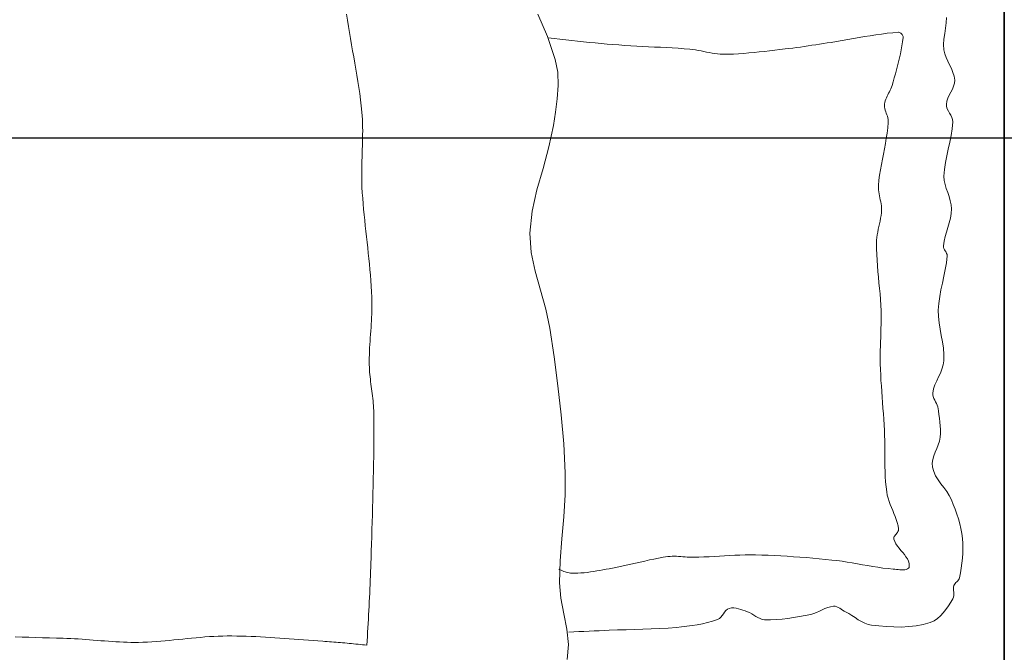
# Model space of a CAD drawing. Units: inches. Extents: x 1484 to 2008, y 1843 to 2590.
# Tile 6 of 21: x 1853 to 1891, y 1981 to 2005. Entities that reach past the tile are written whole.
import ezdxf

# ---------------------------------------------------------------- set-up
doc = ezdxf.new("R2010")
doc.units = ezdxf.units.IN
for name, color, linetype, lineweight in [('A-ANNO-DIMS', 2, 'Continuous', 18), ('A-FURN', 8, 'Continuous', 18), ('A-WALL', 7, 'Continuous', 35)]:
    doc.layers.add(name, color=color, linetype=linetype, lineweight=lineweight)
doc.styles.get("Standard").update_dxf_attribs({"font": 'arial.ttf'})
doc.dimstyles.new('ISO-25', dxfattribs={"dimtxt": 7, "dimasz": 2.5, "dimexe": 1.25, "dimexo": 0.625, "dimtad": 1, "dimdec": 0, "dimlunit": 3, "dimtxsty": 'Standard', "dimcen": 2.5, "dimadec": 0, "dimazin": 0, "dimtfac": 1, "dimtdec": 0, "dimtmove": 0, "dimatfit": 3, "dimfxl": 1, "dimarcsym": 0})

# ---------------------------------------------------------------- blocks, each defined once
blk = doc.blocks.new('BED-DOUBLE')
for p, q in [((48.589, 84.891), (48.4, 84.837)), ((48.78, 84.936), (48.589, 84.891)), ((48.973, 84.972), (48.78, 84.936)), ((49.167, 84.998), (48.973, 84.972)), ((49.359, 85.013), (49.167, 84.998)), ((49.551, 85.017), (49.359, 85.013)), ((49.744, 85.011), (49.551, 85.017)), ((49.937, 84.997), (49.744, 85.011)), ((50.129, 84.977), (49.937, 84.997)), ((50.321, 84.951), (50.129, 84.977)), ((50.512, 84.921), (50.321, 84.951)), ((50.702, 84.887), (50.512, 84.921)), ((50.746, 84.873), (50.702, 84.887)), ((50.784, 84.848), (50.746, 84.873)), ((50.82, 84.817), (50.784, 84.848)), ((30.689, 84.496), (30.546, 84.424)), ((30.832, 84.567), (30.689, 84.496)), ((30.977, 84.628), (30.832, 84.567)), ((31.125, 84.673), (30.977, 84.628)), ((31.278, 84.695), (31.125, 84.673)), ((31.401, 84.686), (31.278, 84.695)), ((31.52, 84.653), (31.401, 84.686)), ((31.637, 84.603), (31.52, 84.653)), ((31.752, 84.545), (31.637, 84.603)), ((31.867, 84.485), (31.752, 84.545)), ((31.984, 84.431), (31.867, 84.485)), ((32.569, 84.494), (32.485, 84.447)), ((32.652, 84.541), (32.569, 84.494)), ((32.736, 84.582), (32.652, 84.541)), ((32.822, 84.61), (32.736, 84.582)), ((32.912, 84.619), (32.822, 84.61)), ((33.179, 84.598), (32.912, 84.619)), ((33.443, 84.556), (33.179, 84.598)), ((33.707, 84.502), (33.443, 84.556)), ((33.97, 84.442), (33.707, 84.502)), ((35.826, 84.476), (35.668, 84.421)), ((35.985, 84.524), (35.826, 84.476)), ((36.145, 84.558), (35.985, 84.524)), ((36.307, 84.57), (36.145, 84.558)), ((36.49, 84.557), (36.307, 84.57)), ((36.671, 84.526), (36.49, 84.557)), ((36.85, 84.482), (36.671, 84.526)), ((37.029, 84.43), (36.85, 84.482)), ((47.495, 84.483), (47.337, 84.382)), ((47.661, 84.566), (47.495, 84.483)), ((47.843, 84.64), (47.661, 84.566)), ((48.027, 84.711), (47.843, 84.64)), ((48.212, 84.777), (48.027, 84.711)), ((48.4, 84.837), (48.212, 84.777)), ((50.855, 84.782), (50.82, 84.817)), ((50.889, 84.745), (50.855, 84.782)), ((50.924, 84.712), (50.889, 84.745)), ((50.962, 84.684), (50.924, 84.712)), ((51.004, 84.664), (50.962, 84.684)), ((51.067, 84.651), (51.004, 84.664)), ((51.133, 84.649), (51.067, 84.651)), ((51.2, 84.654), (51.133, 84.649)), ((51.267, 84.661), (51.2, 84.654)), ((51.334, 84.665), (51.267, 84.661)), ((51.398, 84.664), (51.334, 84.665)), ((51.459, 84.653), (51.398, 84.664)), ((51.516, 84.627), (51.459, 84.653)), ((51.654, 84.54), (51.516, 84.627)), ((51.794, 84.449), (51.654, 84.54)), ((29.039, 84.367), (28.83, 84.378)), ((29.252, 84.339), (29.039, 84.367)), ((29.466, 84.304), (29.252, 84.339)), ((29.68, 84.274), (29.466, 84.304)), ((29.893, 84.259), (29.68, 84.274)), ((30.102, 84.27), (29.893, 84.259)), ((30.254, 84.304), (30.102, 84.27)), ((30.402, 84.358), (30.254, 84.304)), ((30.546, 84.424), (30.402, 84.358)), ((32.103, 84.39), (31.984, 84.431)), ((32.226, 84.372), (32.103, 84.39)), ((32.315, 84.379), (32.226, 84.372)), ((32.401, 84.407), (32.315, 84.379)), ((32.485, 84.447), (32.401, 84.407)), ((34.233, 84.382), (33.97, 84.442)), ((34.497, 84.33), (34.233, 84.382)), ((34.762, 84.292), (34.497, 84.33)), ((35.029, 84.275), (34.762, 84.292)), ((35.192, 84.286), (35.029, 84.275)), ((35.352, 84.319), (35.192, 84.286)), ((35.511, 84.366), (35.352, 84.319)), ((35.668, 84.421), (35.511, 84.366)), ((37.207, 84.376), (37.029, 84.43)), ((37.386, 84.326), (37.207, 84.376)), ((37.566, 84.285), (37.386, 84.326)), ((37.749, 84.259), (37.566, 84.285)), ((37.8, 84.262), (37.749, 84.259)), ((37.849, 84.277), (37.8, 84.262)), ((37.897, 84.301), (37.849, 84.277)), ((37.945, 84.329), (37.897, 84.301)), ((37.992, 84.357), (37.945, 84.329)), ((38.04, 84.381), (37.992, 84.357)), ((38.09, 84.397), (38.04, 84.381)), ((38.141, 84.4), (38.09, 84.397)), ((38.407, 84.37), (38.141, 84.4)), ((38.672, 84.325), (38.407, 84.37)), ((38.936, 84.272), (38.672, 84.325)), ((39.199, 84.215), (38.936, 84.272)), ((39.462, 84.16), (39.199, 84.215)), ((39.726, 84.112), (39.462, 84.16)), ((39.991, 84.075), (39.726, 84.112)), ((40.258, 84.056), (39.991, 84.075)), ((40.753, 84.087), (40.506, 84.061)), ((40.999, 84.126), (40.753, 84.087)), ((41.245, 84.171), (40.999, 84.126)), ((41.491, 84.216), (41.245, 84.171)), ((41.737, 84.252), (41.491, 84.216)), ((41.984, 84.272), (41.737, 84.252)), ((42.231, 84.269), (41.984, 84.272)), ((42.394, 84.244), (42.231, 84.269)), ((42.553, 84.197), (42.394, 84.244)), ((42.709, 84.135), (42.553, 84.197)), ((42.863, 84.064), (42.709, 84.135)), ((44.327, 84.08), (44.179, 84.057)), ((44.475, 84.101), (44.327, 84.08)), ((44.623, 84.118), (44.475, 84.101)), ((44.772, 84.13), (44.623, 84.118)), ((44.92, 84.137), (44.772, 84.13)), ((45.069, 84.136), (44.92, 84.137)), ((45.217, 84.128), (45.069, 84.136)), ((45.365, 84.102), (45.217, 84.128)), ((45.511, 84.056), (45.365, 84.102)), ((47.031, 84.157), (46.877, 84.048)), ((47.183, 84.271), (47.031, 84.157)), ((47.337, 84.382), (47.183, 84.271)), ((51.933, 84.353), (51.794, 84.449)), ((52.065, 84.251), (51.933, 84.353)), ((52.187, 84.141), (52.065, 84.251)), ((52.294, 84.02), (52.187, 84.141)), ((40.506, 84.061), (40.258, 84.056)), ((43.017, 83.992), (42.863, 84.064)), ((43.173, 83.926), (43.017, 83.992)), ((43.331, 83.872), (43.173, 83.926)), ((43.493, 83.838), (43.331, 83.872)), ((43.563, 83.838), (43.493, 83.838)), ((43.631, 83.854), (43.563, 83.838)), ((43.698, 83.881), (43.631, 83.854)), ((43.763, 83.914), (43.698, 83.881)), ((43.829, 83.951), (43.763, 83.914)), ((43.896, 83.986), (43.829, 83.951)), ((43.963, 84.014), (43.896, 83.986)), ((44.033, 84.033), (43.963, 84.014)), ((44.179, 84.057), (44.033, 84.033)), ((45.655, 83.998), (45.511, 84.056)), ((45.799, 83.937), (45.655, 83.998)), ((45.942, 83.881), (45.799, 83.937)), ((46.086, 83.839), (45.942, 83.881)), ((46.231, 83.818), (46.086, 83.839)), ((46.378, 83.826), (46.231, 83.818)), ((46.554, 83.875), (46.378, 83.826)), ((46.719, 83.952), (46.554, 83.875)), ((46.877, 84.048), (46.719, 83.952)), ((52.381, 83.888), (52.294, 84.02)), ((52.444, 83.743), (52.381, 83.888)), ((52.52, 83.468), (52.444, 83.743)), ((52.573, 83.186), (52.52, 83.468)), ((50.149, 82.915), (50.247, 82.924)), ((50.247, 82.924), (50.294, 82.915)), ((52.606, 82.9), (52.573, 83.186)), ((29.413, 82.522), (29.419, 82.546)), ((29.419, 82.546), (29.429, 82.569)), ((29.429, 82.569), (29.443, 82.591)), ((29.443, 82.591), (29.46, 82.612)), ((29.46, 82.612), (29.48, 82.631)), ((29.48, 82.631), (29.502, 82.648)), ((29.502, 82.648), (29.525, 82.662)), ((29.525, 82.662), (29.549, 82.674)), ((29.549, 82.674), (29.574, 82.681)), ((29.574, 82.681), (29.598, 82.685)), ((29.598, 82.685), (29.622, 82.685)), ((29.622, 82.685), (29.781, 82.664)), ((29.781, 82.664), (29.939, 82.639)), ((29.939, 82.639), (30.096, 82.61)), ((30.096, 82.61), (30.253, 82.578)), ((30.253, 82.578), (30.409, 82.543)), ((30.409, 82.543), (30.565, 82.506)), ((49.548, 82.528), (49.631, 82.597)), ((49.631, 82.597), (49.713, 82.667)), ((49.713, 82.667), (49.796, 82.734)), ((49.796, 82.734), (49.88, 82.795)), ((49.88, 82.795), (49.966, 82.848)), ((49.966, 82.848), (50.055, 82.889)), ((50.055, 82.889), (50.149, 82.915)), ((50.294, 82.915), (50.33, 82.891)), ((50.33, 82.891), (50.357, 82.854)), ((50.357, 82.854), (50.374, 82.807)), ((50.374, 82.807), (50.385, 82.751)), ((50.386, 82.555), (50.38, 82.486)), ((50.385, 82.751), (50.39, 82.689)), ((50.39, 82.623), (50.386, 82.555)), ((50.39, 82.689), (50.39, 82.623)), ((52.621, 82.611), (52.606, 82.9)), ((52.62, 82.321), (52.621, 82.611)), ((29.412, 82.499), (29.413, 82.522)), ((29.429, 82.278), (29.412, 82.499)), ((29.452, 82.058), (29.429, 82.278)), ((30.565, 82.506), (30.721, 82.466)), ((30.721, 82.466), (30.876, 82.425)), ((30.876, 82.425), (31.031, 82.383)), ((31.031, 82.383), (31.186, 82.34)), ((31.186, 82.34), (31.34, 82.296)), ((31.34, 82.296), (31.494, 82.253)), ((31.494, 82.253), (31.556, 82.233)), ((31.556, 82.233), (31.616, 82.208)), ((31.616, 82.208), (31.675, 82.181)), ((31.675, 82.181), (31.733, 82.151)), ((47.717, 82.138), (47.836, 82.181)), ((47.836, 82.181), (47.954, 82.228)), ((47.954, 82.228), (48.072, 82.276)), ((48.072, 82.276), (48.189, 82.325)), ((48.189, 82.325), (48.307, 82.372)), ((48.307, 82.372), (48.426, 82.415)), ((48.426, 82.415), (48.546, 82.454)), ((48.546, 82.454), (48.667, 82.486)), ((48.667, 82.486), (48.791, 82.509)), ((48.791, 82.509), (48.827, 82.509)), ((48.827, 82.509), (48.861, 82.5)), ((48.861, 82.5), (48.895, 82.483)), ((48.895, 82.483), (48.928, 82.461)), ((48.928, 82.461), (48.96, 82.435)), ((48.96, 82.435), (48.992, 82.408)), ((48.992, 82.408), (49.024, 82.381)), ((49.024, 82.381), (49.057, 82.357)), ((49.057, 82.357), (49.089, 82.336)), ((49.089, 82.336), (49.122, 82.323)), ((49.122, 82.323), (49.156, 82.317)), ((49.156, 82.317), (49.191, 82.321)), ((49.191, 82.321), (49.286, 82.356)), ((49.286, 82.356), (49.376, 82.405)), ((49.376, 82.405), (49.463, 82.463)), ((49.463, 82.463), (49.548, 82.528)), ((50.361, 82.3), (50.343, 82.099)), ((50.367, 82.357), (50.361, 82.3)), ((50.373, 82.419), (50.367, 82.357)), ((50.38, 82.486), (50.373, 82.419)), ((52.606, 82.03), (52.62, 82.321)), ((29.48, 81.839), (29.452, 82.058)), ((29.511, 81.62), (29.48, 81.839)), ((31.733, 82.151), (31.791, 82.12)), ((31.791, 82.12), (31.849, 82.088)), ((31.849, 82.088), (31.907, 82.058)), ((31.907, 82.058), (31.966, 82.03)), ((31.966, 82.03), (32.025, 82.004)), ((32.025, 82.004), (32.085, 81.983)), ((32.085, 81.983), (32.147, 81.967)), ((32.147, 81.967), (32.21, 81.957)), ((32.21, 81.957), (32.271, 81.955)), ((32.271, 81.955), (32.331, 81.961)), ((32.331, 81.961), (32.392, 81.972)), ((32.392, 81.972), (32.451, 81.989)), ((32.451, 81.989), (32.511, 82.008)), ((32.511, 82.008), (32.571, 82.029)), ((32.571, 82.029), (32.63, 82.05)), ((32.63, 82.05), (32.69, 82.07)), ((32.69, 82.07), (32.75, 82.087)), ((32.75, 82.087), (32.81, 82.1)), ((32.81, 82.1), (32.871, 82.107)), ((32.871, 82.107), (32.932, 82.106)), ((32.932, 82.106), (33.138, 82.087)), ((33.138, 82.087), (33.345, 82.061)), ((33.345, 82.061), (33.55, 82.029)), ((33.55, 82.029), (33.755, 81.994)), ((33.755, 81.994), (33.96, 81.955)), ((33.96, 81.955), (34.164, 81.915)), ((34.164, 81.915), (34.369, 81.875)), ((34.369, 81.875), (34.573, 81.836)), ((34.573, 81.836), (34.778, 81.8)), ((34.778, 81.8), (34.983, 81.768)), ((34.983, 81.768), (35.189, 81.741)), ((35.793, 81.76), (35.872, 81.777)), ((35.872, 81.777), (35.952, 81.795)), ((35.952, 81.795), (36.031, 81.811)), ((36.031, 81.811), (36.11, 81.826)), ((36.11, 81.826), (36.19, 81.837)), ((36.19, 81.837), (36.269, 81.843)), ((36.269, 81.843), (36.349, 81.844)), ((36.349, 81.844), (36.458, 81.837)), ((36.458, 81.837), (36.565, 81.824)), ((36.565, 81.824), (36.673, 81.806)), ((36.673, 81.806), (36.78, 81.786)), ((36.78, 81.786), (36.887, 81.763)), ((39.405, 81.764), (39.625, 81.784)), ((39.625, 81.784), (39.846, 81.801)), ((39.846, 81.801), (40.067, 81.815)), ((40.067, 81.815), (40.288, 81.824)), ((40.288, 81.824), (40.46, 81.828)), ((40.46, 81.828), (40.631, 81.828)), ((40.631, 81.828), (40.803, 81.825)), ((40.803, 81.825), (40.975, 81.821)), ((40.975, 81.821), (41.147, 81.815)), ((41.147, 81.815), (41.318, 81.809)), ((41.318, 81.809), (41.49, 81.802)), ((41.49, 81.802), (41.662, 81.797)), ((41.662, 81.797), (41.834, 81.792)), ((41.834, 81.792), (42.005, 81.789)), ((42.005, 81.789), (42.177, 81.789)), ((42.177, 81.789), (42.349, 81.792)), ((42.349, 81.792), (42.566, 81.799)), ((42.566, 81.799), (42.782, 81.809)), ((42.782, 81.809), (42.999, 81.821)), ((42.999, 81.821), (43.216, 81.835)), ((43.216, 81.835), (43.432, 81.85)), ((43.432, 81.85), (43.649, 81.866)), ((43.649, 81.866), (43.865, 81.882)), ((43.865, 81.882), (44.082, 81.898)), ((44.082, 81.898), (44.298, 81.914)), ((44.298, 81.914), (44.515, 81.928)), ((44.515, 81.928), (44.732, 81.942)), ((44.732, 81.942), (44.948, 81.954)), ((44.948, 81.954), (45.149, 81.962)), ((45.149, 81.962), (45.349, 81.967)), ((45.349, 81.967), (45.55, 81.969)), ((45.55, 81.969), (45.751, 81.97)), ((45.751, 81.97), (45.952, 81.971)), ((45.952, 81.971), (46.153, 81.972)), ((46.153, 81.972), (46.354, 81.975)), ((46.354, 81.975), (46.554, 81.98)), ((46.554, 81.98), (46.754, 81.989)), ((46.754, 81.989), (46.954, 82.002)), ((46.954, 82.002), (47.153, 82.02)), ((47.153, 82.02), (47.352, 82.046)), ((47.352, 82.046), (47.476, 82.068)), ((47.476, 82.068), (47.597, 82.1)), ((47.597, 82.1), (47.717, 82.138)), ((50.319, 81.899), (50.291, 81.699)), ((50.343, 82.099), (50.319, 81.899)), ((52.581, 81.741), (52.606, 82.03)), ((29.545, 81.401), (29.511, 81.62)), ((29.582, 81.182), (29.545, 81.401)), ((35.189, 81.741), (35.396, 81.722)), ((35.396, 81.722), (35.476, 81.719)), ((35.476, 81.719), (35.555, 81.723)), ((35.555, 81.723), (35.635, 81.732)), ((35.635, 81.732), (35.714, 81.745)), ((35.714, 81.745), (35.793, 81.76)), ((36.887, 81.763), (36.994, 81.739)), ((36.994, 81.739), (37.101, 81.716)), ((37.101, 81.716), (37.208, 81.694)), ((37.208, 81.694), (37.315, 81.674)), ((37.315, 81.674), (37.423, 81.659)), ((37.423, 81.659), (37.531, 81.648)), ((37.531, 81.648), (37.639, 81.644)), ((37.639, 81.644), (37.86, 81.646)), ((37.86, 81.646), (38.081, 81.654)), ((38.081, 81.654), (38.302, 81.667)), ((38.302, 81.667), (38.523, 81.683)), ((38.523, 81.683), (38.743, 81.702)), ((38.743, 81.702), (38.964, 81.722)), ((38.964, 81.722), (39.184, 81.743)), ((39.184, 81.743), (39.405, 81.764)), ((50.26, 81.499), (50.226, 81.3)), ((50.291, 81.699), (50.26, 81.499)), ((52.52, 81.317), (52.549, 81.455)), ((52.549, 81.455), (52.581, 81.741)), ((29.62, 80.964), (29.582, 81.182)), ((50.192, 81.1), (50.157, 80.901)), ((50.226, 81.3), (50.192, 81.1)), ((52.335, 80.933), (52.409, 81.057)), ((52.409, 81.057), (52.472, 81.185)), ((52.472, 81.185), (52.52, 81.317)), ((29.659, 80.746), (29.62, 80.964)), ((29.698, 80.527), (29.659, 80.746)), ((50.122, 80.702), (50.089, 80.503)), ((50.157, 80.901), (50.122, 80.702)), ((52.099, 80.564), (52.176, 80.687)), ((52.176, 80.687), (52.256, 80.81)), ((52.256, 80.81), (52.335, 80.933)), ((29.736, 80.309), (29.698, 80.527)), ((29.772, 80.09), (29.736, 80.309)), ((50.058, 80.303), (50.031, 80.103)), ((50.089, 80.503), (50.058, 80.303)), ((51.887, 80.211), (51.924, 80.267)), ((51.924, 80.267), (51.962, 80.324)), ((51.962, 80.324), (51.998, 80.38)), ((51.998, 80.38), (52.03, 80.437)), ((52.03, 80.437), (52.099, 80.564)), ((29.806, 79.872), (29.772, 80.09)), ((29.828, 79.723), (29.806, 79.872)), ((50.008, 79.902), (49.983, 79.654)), ((50.031, 80.103), (50.008, 79.902)), ((51.811, 79.971), (51.813, 80.034)), ((51.828, 79.856), (51.811, 79.971)), ((51.813, 80.034), (51.829, 80.094)), ((51.861, 79.744), (51.828, 79.856)), ((51.829, 80.094), (51.854, 80.153)), ((51.854, 80.153), (51.887, 80.211)), ((29.851, 79.574), (29.828, 79.723)), ((29.874, 79.425), (29.851, 79.574)), ((49.983, 79.654), (49.959, 79.407)), ((51.905, 79.636), (51.861, 79.744)), ((51.956, 79.528), (51.905, 79.636)), ((52.008, 79.42), (51.956, 79.528)), ((29.897, 79.276), (29.874, 79.425)), ((29.92, 79.127), (29.897, 79.276)), ((29.943, 78.978), (29.92, 79.127)), ((49.937, 79.159), (49.915, 78.911)), ((49.959, 79.407), (49.937, 79.159)), ((52.057, 79.312), (52.008, 79.42)), ((52.099, 79.202), (52.057, 79.312)), ((52.129, 79.089), (52.099, 79.202)), ((52.172, 78.865), (52.129, 79.089)), ((29.965, 78.829), (29.943, 78.978)), ((29.987, 78.679), (29.965, 78.829)), ((49.915, 78.911), (49.896, 78.663)), ((52.214, 78.64), (52.172, 78.865)), ((30.008, 78.53), (29.987, 78.679)), ((30.027, 78.381), (30.008, 78.53)), ((30.046, 78.231), (30.027, 78.381)), ((49.877, 78.414), (49.861, 78.166)), ((49.896, 78.663), (49.877, 78.414)), ((52.253, 78.415), (52.214, 78.64)), ((52.286, 78.189), (52.253, 78.415)), ((30.063, 78.082), (30.046, 78.231)), ((30.086, 77.881), (30.063, 78.082)), ((49.861, 78.166), (49.846, 77.917)), ((52.313, 77.962), (52.286, 78.189)), ((52.332, 77.735), (52.313, 77.962)), ((30.11, 77.68), (30.086, 77.881)), ((30.133, 77.479), (30.11, 77.68)), ((49.834, 77.669), (49.823, 77.42)), ((49.846, 77.917), (49.834, 77.669)), ((52.341, 77.508), (52.332, 77.735)), ((30.156, 77.277), (30.133, 77.479)), ((30.179, 77.076), (30.156, 77.277)), ((49.815, 77.172), (49.808, 76.923)), ((49.823, 77.42), (49.815, 77.172)), ((52.295, 77.106), (52.324, 77.192)), ((52.324, 77.192), (52.337, 77.281)), ((52.337, 77.281), (52.341, 77.508)), ((30.2, 76.875), (30.179, 77.076)), ((30.219, 76.673), (30.2, 76.875)), ((49.808, 76.923), (49.807, 76.722)), ((52.059, 76.7), (52.103, 76.783)), ((52.103, 76.783), (52.154, 76.863)), ((52.154, 76.863), (52.205, 76.943)), ((52.205, 76.943), (52.254, 77.024)), ((52.254, 77.024), (52.295, 77.106)), ((30.236, 76.472), (30.219, 76.673)), ((30.25, 76.27), (30.236, 76.472)), ((49.807, 76.722), (49.809, 76.522)), ((49.809, 76.522), (49.814, 76.322)), ((51.934, 76.35), (51.964, 76.439)), ((51.964, 76.439), (51.995, 76.527)), ((51.995, 76.527), (52.024, 76.614)), ((52.024, 76.614), (52.059, 76.7)), ((30.261, 76.068), (30.25, 76.27)), ((30.268, 75.866), (30.261, 76.068)), ((49.814, 76.322), (49.822, 76.122)), ((49.822, 76.122), (49.831, 75.921)), ((51.877, 76.08), (51.888, 76.17)), ((51.878, 75.991), (51.877, 76.08)), ((51.888, 76.17), (51.908, 76.26)), ((51.908, 76.26), (51.934, 76.35)), ((30.271, 75.664), (30.268, 75.866)), ((30.268, 75.556), (30.271, 75.664)), ((49.831, 75.921), (49.842, 75.721)), ((49.842, 75.721), (49.854, 75.521)), ((51.893, 75.902), (51.878, 75.991)), ((51.925, 75.833), (51.893, 75.902)), ((51.974, 75.774), (51.925, 75.833)), ((52.037, 75.723), (51.974, 75.774)), ((52.106, 75.675), (52.037, 75.723)), ((52.176, 75.628), (52.106, 75.675)), ((52.241, 75.577), (52.176, 75.628)), ((30.228, 75.233), (30.245, 75.34)), ((30.245, 75.34), (30.259, 75.448)), ((30.259, 75.448), (30.268, 75.556)), ((49.854, 75.521), (49.866, 75.32)), ((49.866, 75.32), (49.877, 75.12)), ((52.295, 75.519), (52.241, 75.577)), ((52.333, 75.452), (52.295, 75.519)), ((52.397, 75.258), (52.333, 75.452)), ((52.45, 75.06), (52.397, 75.258)), ((30.14, 74.805), (30.163, 74.912)), ((30.163, 74.912), (30.186, 75.019)), ((30.186, 75.019), (30.208, 75.126)), ((30.208, 75.126), (30.228, 75.233)), ((49.877, 75.12), (49.887, 74.92)), ((49.887, 74.92), (49.895, 74.72)), ((52.496, 74.861), (52.45, 75.06)), ((52.533, 74.659), (52.496, 74.861)), ((30.071, 74.374), (30.083, 74.482)), ((30.083, 74.482), (30.1, 74.59)), ((30.1, 74.59), (30.119, 74.697)), ((30.119, 74.697), (30.14, 74.805)), ((49.895, 74.72), (49.9, 74.519)), ((49.9, 74.519), (49.9, 74.435)), ((52.565, 74.456), (52.533, 74.659)), ((30.036, 73.913), (30.052, 74.144)), ((30.052, 74.144), (30.071, 74.374)), ((49.88, 74.099), (49.873, 74.015)), ((49.887, 74.183), (49.88, 74.099)), ((49.893, 74.267), (49.887, 74.183)), ((49.897, 74.351), (49.893, 74.267)), ((49.9, 74.435), (49.897, 74.351)), ((52.592, 74.252), (52.565, 74.456)), ((52.615, 74.048), (52.592, 74.252)), ((30.021, 73.682), (30.036, 73.913)), ((49.863, 73.847), (49.861, 73.764)), ((49.861, 73.764), (49.862, 73.68)), ((49.868, 73.931), (49.863, 73.847)), ((49.873, 74.015), (49.868, 73.931)), ((52.635, 73.844), (52.615, 74.048)), ((52.663, 73.518), (52.635, 73.844)), ((29.997, 73.219), (30.009, 73.451)), ((30.009, 73.451), (30.021, 73.682)), ((49.862, 73.68), (49.866, 73.597)), ((49.866, 73.597), (49.875, 73.513)), ((49.875, 73.513), (49.902, 73.331)), ((49.902, 73.331), (49.933, 73.15)), ((52.684, 73.191), (52.663, 73.518)), ((29.976, 72.757), (29.987, 72.988)), ((29.987, 72.988), (29.997, 73.219)), ((49.933, 73.15), (49.968, 72.969)), ((49.968, 72.969), (50.006, 72.789)), ((52.699, 72.864), (52.684, 73.191)), ((29.965, 72.526), (29.976, 72.757)), ((50.006, 72.789), (50.046, 72.609)), ((50.046, 72.609), (50.087, 72.429)), ((52.71, 72.537), (52.699, 72.864)), ((29.94, 72.063), (29.953, 72.295)), ((29.953, 72.295), (29.965, 72.526)), ((50.087, 72.429), (50.129, 72.25)), ((50.129, 72.25), (50.171, 72.07)), ((52.718, 72.209), (52.71, 72.537)), ((52.727, 71.882), (52.718, 72.209)), ((29.908, 71.602), (29.925, 71.833)), ((29.925, 71.833), (29.94, 72.063)), ((50.171, 72.07), (50.212, 71.891)), ((50.212, 71.891), (50.252, 71.711)), ((52.736, 71.554), (52.727, 71.882)), ((29.889, 71.371), (29.908, 71.602)), ((50.252, 71.711), (50.289, 71.53)), ((50.289, 71.53), (50.323, 71.349)), ((52.749, 71.227), (52.736, 71.554)), ((29.849, 70.911), (29.87, 71.141)), ((29.87, 71.141), (29.889, 71.371)), ((50.323, 71.349), (50.345, 71.227)), ((50.345, 71.227), (50.368, 71.104)), ((50.368, 71.104), (50.39, 70.982)), ((52.757, 71.029), (52.749, 71.227)), ((52.766, 70.832), (52.757, 71.029)), ((29.806, 70.451), (29.828, 70.681)), ((29.828, 70.681), (29.849, 70.911)), ((50.39, 70.982), (50.412, 70.859)), ((50.412, 70.859), (50.433, 70.736)), ((50.433, 70.736), (50.453, 70.613)), ((52.775, 70.634), (52.766, 70.832)), ((29.783, 70.221), (29.806, 70.451)), ((50.453, 70.613), (50.471, 70.49)), ((50.471, 70.49), (50.488, 70.366)), ((50.488, 70.366), (50.501, 70.243)), ((52.784, 70.437), (52.775, 70.634)), ((52.793, 70.239), (52.784, 70.437)), ((29.735, 69.761), (29.76, 69.991)), ((29.76, 69.991), (29.783, 70.221)), ((50.501, 70.243), (50.512, 70.119)), ((50.512, 70.119), (50.52, 69.995)), ((50.52, 69.995), (50.524, 69.871)), ((50.524, 69.871), (50.524, 69.818)), ((52.802, 70.042), (52.793, 70.239)), ((52.811, 69.844), (52.802, 70.042)), ((29.684, 69.302), (29.71, 69.532)), ((29.71, 69.532), (29.735, 69.761)), ((46.611, 69.512), (45.475, 69.449)), ((47.469, 69.508), (46.611, 69.512)), ((48.327, 69.451), (47.469, 69.508)), ((50.468, 69.501), (50.45, 69.45)), ((50.483, 69.552), (50.468, 69.501)), ((50.496, 69.605), (50.483, 69.552)), ((50.507, 69.658), (50.496, 69.605)), ((50.515, 69.711), (50.507, 69.658)), ((50.521, 69.764), (50.515, 69.711)), ((50.524, 69.818), (50.521, 69.764)), ((52.703, 69.567), (52.103, 69.452)), ((53.299, 69.631), (52.703, 69.567)), ((52.82, 69.647), (52.811, 69.844)), ((53.892, 69.59), (53.299, 69.631)), ((30.471, 69.119), (29.579, 68.813)), ((29.657, 69.072), (29.684, 69.302)), ((30.973, 69.217), (30.471, 69.119)), ((31.488, 69.235), (30.973, 69.217)), ((32.008, 69.198), (31.488, 69.235)), ((32.529, 69.128), (32.008, 69.198)), ((33.044, 69.05), (32.529, 69.128)), ((43.211, 69.223), (42.083, 69.075)), ((44.342, 69.35), (43.211, 69.223)), ((45.475, 69.449), (44.342, 69.35)), ((49.184, 69.375), (48.327, 69.451)), ((50.042, 69.309), (49.184, 69.375)), ((50.901, 69.287), (50.042, 69.309)), ((50.384, 69.303), (50.358, 69.257)), ((50.408, 69.351), (50.384, 69.303)), ((50.431, 69.4), (50.408, 69.351)), ((50.45, 69.45), (50.431, 69.4)), ((51.502, 69.34), (50.901, 69.287)), ((52.103, 69.452), (51.502, 69.34)), ((29.579, 68.813), (28.71, 68.44)), ((29.629, 68.843), (29.657, 69.072)), ((33.889, 68.877), (33.044, 69.05)), ((34.725, 68.644), (33.889, 68.877)), ((40.213, 68.759), (39.476, 68.552)), ((40.957, 68.913), (40.213, 68.759)), ((42.083, 69.075), (40.957, 68.913)), ((35.559, 68.405), (34.725, 68.644)), ((36.399, 68.216), (35.559, 68.405)), ((38.741, 68.343), (38.002, 68.186)), ((39.476, 68.552), (38.741, 68.343)), ((37.252, 68.131), (36.399, 68.216)), ((38.002, 68.186), (37.252, 68.131)), ((37.818, 61.809), (37.604, 61.785)), ((38.032, 61.832), (37.818, 61.809)), ((38.247, 61.855), (38.032, 61.832)), ((38.461, 61.876), (38.247, 61.855)), ((38.675, 61.897), (38.461, 61.876)), ((38.89, 61.915), (38.675, 61.897)), ((39.105, 61.933), (38.89, 61.915)), ((39.32, 61.948), (39.105, 61.933)), ((39.535, 61.96), (39.32, 61.948)), ((39.75, 61.971), (39.535, 61.96)), ((39.882, 61.975), (39.75, 61.971)), ((40.014, 61.976), (39.882, 61.975)), ((40.146, 61.975), (40.014, 61.976)), ((40.277, 61.973), (40.146, 61.975)), ((40.409, 61.968), (40.277, 61.973)), ((40.541, 61.962), (40.409, 61.968)), ((40.673, 61.955), (40.541, 61.962)), ((40.805, 61.946), (40.673, 61.955)), ((40.937, 61.938), (40.805, 61.946)), ((41.069, 61.928), (40.937, 61.938)), ((41.201, 61.919), (41.069, 61.928)), ((41.333, 61.909), (41.201, 61.919)), ((41.465, 61.9), (41.333, 61.909)), ((41.597, 61.892), (41.465, 61.9)), ((41.729, 61.885), (41.597, 61.892)), ((41.861, 61.878), (41.729, 61.885)), ((41.993, 61.873), (41.861, 61.878)), ((42.125, 61.87), (41.993, 61.873)), ((42.257, 61.869), (42.125, 61.87)), ((42.389, 61.87), (42.257, 61.869)), ((42.483, 61.873), (42.389, 61.87)), ((42.577, 61.878), (42.483, 61.873)), ((42.671, 61.884), (42.577, 61.878)), ((42.764, 61.892), (42.671, 61.884)), ((42.858, 61.902), (42.764, 61.892)), ((42.952, 61.912), (42.858, 61.902)), ((43.045, 61.923), (42.952, 61.912)), ((43.139, 61.936), (43.045, 61.923)), ((43.232, 61.948), (43.139, 61.936)), ((43.326, 61.961), (43.232, 61.948)), ((43.419, 61.973), (43.326, 61.961)), ((43.513, 61.986), (43.419, 61.973)), ((43.606, 61.998), (43.513, 61.986)), ((43.7, 62.009), (43.606, 61.998)), ((43.794, 62.019), (43.7, 62.009)), ((43.887, 62.028), (43.794, 62.019)), ((43.981, 62.036), (43.887, 62.028)), ((44.075, 62.041), (43.981, 62.036)), ((44.169, 62.046), (44.075, 62.041)), ((44.263, 62.048), (44.169, 62.046)), ((44.547, 62.05), (44.263, 62.048)), ((44.832, 62.05), (44.547, 62.05)), ((45.116, 62.05), (44.832, 62.05)), ((45.401, 62.048), (45.116, 62.05)), ((45.685, 62.046), (45.401, 62.048)), ((45.97, 62.042), (45.685, 62.046)), ((46.254, 62.038), (45.97, 62.042)), ((46.538, 62.033), (46.254, 62.038)), ((46.823, 62.027), (46.538, 62.033)), ((47.107, 62.021), (46.823, 62.027)), ((47.392, 62.014), (47.107, 62.021)), ((47.676, 62.007), (47.392, 62.014)), ((47.96, 61.999), (47.676, 62.007)), ((48.245, 61.991), (47.96, 61.999)), ((48.529, 61.982), (48.245, 61.991)), ((48.814, 61.974), (48.529, 61.982)), ((49.098, 61.965), (48.814, 61.974)), ((49.382, 61.956), (49.098, 61.965)), ((49.667, 61.948), (49.382, 61.956)), ((49.951, 61.939), (49.667, 61.948)), ((50.12, 61.934), (49.951, 61.939)), ((50.289, 61.928), (50.12, 61.934)), ((50.459, 61.922), (50.289, 61.928)), ((50.628, 61.916), (50.459, 61.922)), ((50.797, 61.909), (50.628, 61.916)), ((50.966, 61.903), (50.797, 61.909)), ((51.135, 61.895), (50.966, 61.903)), ((51.304, 61.888), (51.135, 61.895)), ((51.474, 61.88), (51.304, 61.888)), ((51.643, 61.872), (51.474, 61.88)), ((51.812, 61.864), (51.643, 61.872)), ((51.981, 61.855), (51.812, 61.864)), ((52.15, 61.846), (51.981, 61.855)), ((52.319, 61.837), (52.15, 61.846)), ((52.488, 61.827), (52.319, 61.837)), ((52.657, 61.817), (52.488, 61.827)), ((52.826, 61.807), (52.657, 61.817)), ((52.995, 61.796), (52.826, 61.807)), ((31.327, 61.426), (31.089, 61.387)), ((31.566, 61.462), (31.327, 61.426)), ((31.805, 61.496), (31.566, 61.462)), ((32.045, 61.528), (31.805, 61.496)), ((32.285, 61.556), (32.045, 61.528)), ((32.525, 61.58), (32.285, 61.556)), ((32.671, 61.593), (32.525, 61.58)), ((32.817, 61.602), (32.671, 61.593)), ((32.964, 61.608), (32.817, 61.602)), ((33.11, 61.611), (32.964, 61.608)), ((33.257, 61.613), (33.11, 61.611)), ((33.403, 61.612), (33.257, 61.613)), ((33.55, 61.61), (33.403, 61.612)), ((33.697, 61.607), (33.55, 61.61)), ((33.844, 61.603), (33.697, 61.607)), ((33.991, 61.598), (33.844, 61.603)), ((34.137, 61.593), (33.991, 61.598)), ((34.284, 61.588), (34.137, 61.593)), ((34.431, 61.583), (34.284, 61.588)), ((34.578, 61.579), (34.431, 61.583)), ((34.725, 61.576), (34.578, 61.579)), ((34.872, 61.574), (34.725, 61.576)), ((35.018, 61.574), (34.872, 61.574)), ((35.165, 61.576), (35.018, 61.574)), ((35.312, 61.579), (35.165, 61.576)), ((35.458, 61.586), (35.312, 61.579)), ((35.673, 61.599), (35.458, 61.586)), ((35.888, 61.614), (35.673, 61.599)), ((36.103, 61.631), (35.888, 61.614)), ((36.317, 61.65), (36.103, 61.631)), ((36.532, 61.67), (36.317, 61.65)), ((36.746, 61.692), (36.532, 61.67)), ((36.961, 61.715), (36.746, 61.692)), ((37.175, 61.738), (36.961, 61.715)), ((37.389, 61.762), (37.175, 61.738)), ((37.604, 61.785), (37.389, 61.762)), ((53.164, 61.785), (52.995, 61.796)), ((53.333, 61.774), (53.164, 61.785)), ((53.286, 61.345), (53.295, 61.431)), ((53.295, 61.431), (53.304, 61.517)), ((53.304, 61.517), (53.314, 61.603)), ((53.314, 61.603), (53.323, 61.688)), ((53.323, 61.688), (53.333, 61.774)), ((29.183, 61.054), (28.945, 61.015)), ((29.421, 61.095), (29.183, 61.054)), ((29.66, 61.136), (29.421, 61.095)), ((29.898, 61.179), (29.66, 61.136)), ((30.136, 61.221), (29.898, 61.179)), ((30.374, 61.264), (30.136, 61.221)), ((30.612, 61.306), (30.374, 61.264)), ((30.85, 61.347), (30.612, 61.306)), ((31.089, 61.387), (30.85, 61.347)), ((53.253, 61.002), (53.261, 61.088)), ((53.261, 61.088), (53.269, 61.174)), ((53.269, 61.174), (53.278, 61.26)), ((53.278, 61.26), (53.286, 61.345)), ((28.945, 61.015), (28.706, 60.978)), ((53.215, 60.573), (53.222, 60.658)), ((53.222, 60.658), (53.229, 60.744)), ((53.229, 60.744), (53.237, 60.83)), ((53.237, 60.83), (53.245, 60.916)), ((53.245, 60.916), (53.253, 61.002)), ((53.189, 60.229), (53.195, 60.315)), ((53.195, 60.315), (53.202, 60.401)), ((53.202, 60.401), (53.208, 60.487)), ((53.208, 60.487), (53.215, 60.573)), ((53.164, 59.87), (53.177, 60.056)), ((53.177, 60.056), (53.183, 60.142)), ((53.183, 60.142), (53.189, 60.229)), ((53.137, 59.497), (53.151, 59.684)), ((53.151, 59.684), (53.164, 59.87)), ((53.095, 58.938), (53.109, 59.125)), ((53.109, 59.125), (53.123, 59.311)), ((53.123, 59.311), (53.137, 59.497)), ((53.067, 58.566), (53.081, 58.752)), ((53.081, 58.752), (53.095, 58.938)), ((53.04, 58.193), (53.053, 58.379)), ((53.053, 58.379), (53.067, 58.566)), ((53.017, 57.82), (53.028, 58.006)), ((53.028, 58.006), (53.04, 58.193)), ((52.997, 57.447), (53.006, 57.633)), ((53.006, 57.633), (53.017, 57.82)), ((52.982, 57.074), (52.989, 57.26)), ((52.989, 57.26), (52.997, 57.447)), ((52.973, 56.701), (52.977, 56.887)), ((52.977, 56.887), (52.982, 57.074)), ((52.971, 56.514), (52.973, 56.701)), ((52.971, 56.327), (52.971, 56.514)), ((52.974, 56.154), (52.971, 56.327)), ((52.979, 55.981), (52.974, 56.154)), ((52.988, 55.808), (52.979, 55.981)), ((52.998, 55.635), (52.988, 55.808)), ((53.011, 55.463), (52.998, 55.635)), ((53.025, 55.29), (53.011, 55.463)), ((53.041, 55.118), (53.025, 55.29)), ((53.057, 54.945), (53.041, 55.118)), ((53.075, 54.772), (53.057, 54.945)), ((53.092, 54.6), (53.075, 54.772)), ((53.11, 54.427), (53.092, 54.6)), ((53.128, 54.255), (53.11, 54.427)), ((53.144, 54.082), (53.128, 54.255)), ((53.161, 53.91), (53.144, 54.082)), ((53.175, 53.737), (53.161, 53.91)), ((53.189, 53.565), (53.175, 53.737)), ((53.2, 53.392), (53.189, 53.565)), ((53.209, 53.219), (53.2, 53.392)), ((53.216, 53.046), (53.209, 53.219)), ((53.22, 52.873), (53.216, 53.046)), ((53.221, 52.726), (53.22, 52.873)), ((53.22, 52.579), (53.221, 52.726)), ((53.205, 52.138), (53.211, 52.285)), ((53.211, 52.285), (53.216, 52.432)), ((53.216, 52.432), (53.22, 52.579)), ((53.178, 51.698), (53.188, 51.844)), ((53.188, 51.844), (53.197, 51.991)), ((53.197, 51.991), (53.205, 52.138)), ((53.156, 51.404), (53.167, 51.551)), ((53.167, 51.551), (53.178, 51.698)), ((53.121, 50.964), (53.133, 51.111)), ((53.133, 51.111), (53.144, 51.257)), ((53.144, 51.257), (53.156, 51.404)), ((53.099, 50.67), (53.11, 50.817)), ((53.11, 50.817), (53.121, 50.964)), ((53.072, 50.23), (53.08, 50.377)), ((53.08, 50.377), (53.089, 50.523)), ((53.089, 50.523), (53.099, 50.67)), ((53.054, 49.669), (53.061, 49.936)), ((53.061, 49.936), (53.066, 50.083)), ((53.066, 50.083), (53.072, 50.23)), ((53.046, 49.402), (53.054, 49.669)), ((53.038, 49.135), (53.046, 49.402)), ((53.023, 48.601), (53.031, 48.868)), ((53.031, 48.868), (53.038, 49.135)), ((53.016, 48.334), (53.023, 48.601)), ((53.009, 48.067), (53.016, 48.334))]:
    blk.add_line(p, q)
blk = doc.blocks.new('*D9')
at = {"layer": 'A-ANNO-DIMS', "color": 0, "lineweight": -2, "transparency": 16777216}
for p, q in [((1804.291, 1973.808), (1804.291, 1960.431)), ((1889.307, 1973.808), (1889.307, 1960.431)), ((1806.791, 1961.681), (1886.807, 1961.681)), ((1889.307, 1961.681), (2001.132, 1961.681))]:
    blk.add_line(p, q, dxfattribs=at)
at = {"layer": 'A-ANNO-DIMS', "color": 0, "transparency": 16777216}
for points in [[(1806.791, 1962.097), (1806.791, 1961.264), (1804.291, 1961.681)], [(1886.807, 1962.097), (1886.807, 1961.264), (1889.307, 1961.681)]]:
    blk.add_solid(points, dxfattribs=at)
at = {"layer": 'Defpoints', "color": 0, "transparency": 16777216}
for p in [(1804.291, 1974.433), (1889.307, 1974.433), (1889.307, 1961.681)]:
    blk.add_point(p, dxfattribs=at)
at = {"layer": 'A-ANNO-DIMS', "color": 0, "transparency": 16777216, "insert": (1946.47, 1965.927), "char_height": 7, "attachment_point": 5}
blk.add_mtext('DOUBLE BED 7\'-1" TYP.', dxfattribs=at)
blk = doc.blocks.new('*D32')
at = {"layer": 'A-ANNO-DIMS', "color": 0, "lineweight": -2, "transparency": 16777216}
for p, q in [((1961.855, 2010.803), (1961.855, 2038.599)), ((1648.545, 2010.803), (1963.105, 2010.803)), ((1961.855, 2003.303), (1961.855, 2008.303)), ((1648.545, 2000.803), (1963.105, 2000.803))]:
    blk.add_line(p, q, dxfattribs=at)
at = {"layer": 'A-ANNO-DIMS', "color": 0, "transparency": 16777216}
for points in [[(1961.438, 2008.303), (1962.271, 2008.303), (1961.855, 2010.803)], [(1961.438, 2003.303), (1962.271, 2003.303), (1961.855, 2000.803)]]:
    blk.add_solid(points, dxfattribs=at)
at = {"layer": 'Defpoints', "color": 0, "transparency": 16777216}
for p in [(1647.92, 2010.803), (1961.855, 2010.803), (1647.92, 2000.803)]:
    blk.add_point(p, dxfattribs=at)
at = {"layer": 'A-ANNO-DIMS', "color": 0, "transparency": 16777216, "insert": (1957.656, 2025.951), "char_height": 7, "attachment_point": 5, "rotation": 90}
blk.add_mtext('0\'-10"', dxfattribs=at)

msp = doc.modelspace()

# ---------------------------------------------------------------- linework, layer by layer
at = {"layer": 'A-WALL'}
msp.add_line((1890.92, 2072.803), (1890.92, 1928.803), dxfattribs=at)

# ---------------------------------------------------------------- block references
at = {"layer": 'A-FURN', "rotation": 269.9999999999906}
msp.add_blockref('BED-DOUBLE', (1804.291, 2034.333), dxfattribs=at)

# ---------------------------------------------------------------- dimensions: what is measured, and where the dimension line sits
at = {"layer": 'A-ANNO-DIMS'}
dim = msp.add_linear_dim(base=(1961.855, 2010.803), p1=(1647.92, 2000.803), p2=(1647.92, 2010.803), angle=90, dimstyle='ISO-25', override={"dimdec": 1, "dimlfac": 1, "dimrnd": 0, "dimzin": 1, "dimdsep": 46, "dimlunit": 4, "dimfrac": 2}, dxfattribs=at)
dim.commit()
dim.dimension.update_dxf_attribs({"geometry": '*D32', "text_midpoint": (1957.656, 2025.951)})
dim = msp.add_linear_dim(base=(1889.307, 1961.681), p1=(1804.291, 1974.433), p2=(1889.307, 1974.433), text='DOUBLE BED <> TYP.', dimstyle='ISO-25', override={"dimdec": 1, "dimlfac": 1, "dimrnd": 0, "dimzin": 1, "dimdsep": 46, "dimlunit": 4, "dimfrac": 2}, dxfattribs=at)
dim.commit()
dim.dimension.update_dxf_attribs({"geometry": '*D9', "text_midpoint": (1946.47, 1965.927)})

doc.saveas('drawing.dxf')
